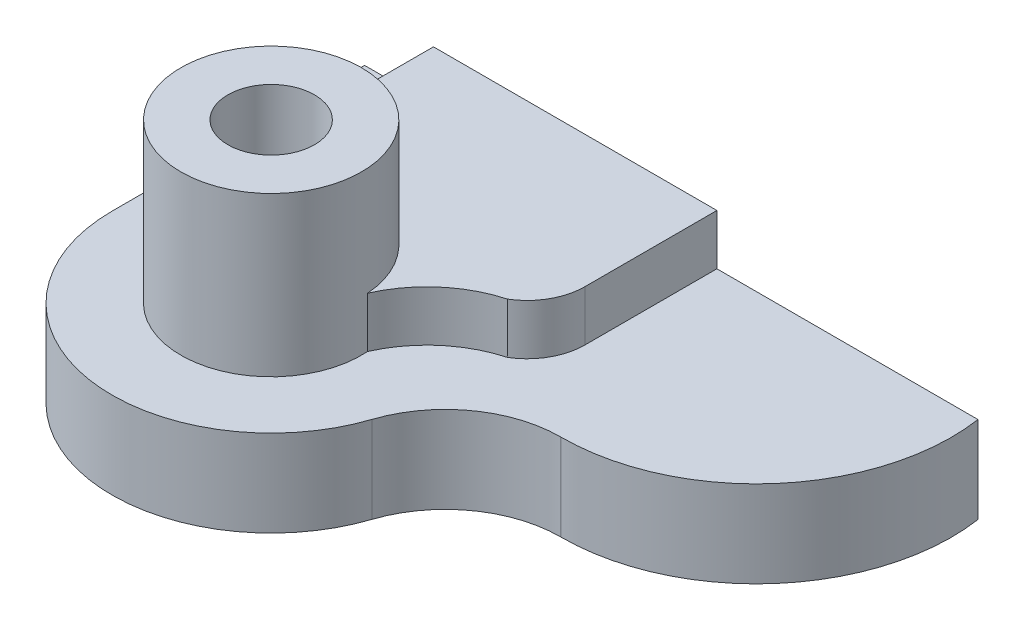
ISO-10303-21;
HEADER;
FILE_DESCRIPTION(('STEP AP214'),'2;1');
FILE_NAME('part.step','',(''),(''),'','','');
FILE_SCHEMA(('AUTOMOTIVE_DESIGN { 1 0 10303 214 1 1 1 1 }'));
ENDSEC;
DATA;
#1=APPLICATION_CONTEXT('core data for automotive mechanical design processes');
#2=APPLICATION_PROTOCOL_DEFINITION('international standard','automotive_design',2000,#1);
#3=PRODUCT_CONTEXT('',#1,'mechanical');
#4=PRODUCT('Part','Part','',(#3));
#5=PRODUCT_RELATED_PRODUCT_CATEGORY('part','',(#4));
#6=PRODUCT_DEFINITION_FORMATION('','',#4);
#7=PRODUCT_DEFINITION_CONTEXT('part definition',#1,'design');
#8=PRODUCT_DEFINITION('design','',#6,#7);
#9=PRODUCT_DEFINITION_SHAPE('','',#8);
#10=(LENGTH_UNIT() NAMED_UNIT(*) SI_UNIT(.MILLI.,.METRE.));
#11=(NAMED_UNIT(*) PLANE_ANGLE_UNIT() SI_UNIT($,.RADIAN.));
#12=(NAMED_UNIT(*) SI_UNIT($,.STERADIAN.) SOLID_ANGLE_UNIT());
#13=UNCERTAINTY_MEASURE_WITH_UNIT(LENGTH_MEASURE(1.E-05),#10,'distance_accuracy_value','');
#14=(GEOMETRIC_REPRESENTATION_CONTEXT(3) GLOBAL_UNCERTAINTY_ASSIGNED_CONTEXT((#13)) GLOBAL_UNIT_ASSIGNED_CONTEXT((#10,
#11,#12)) REPRESENTATION_CONTEXT('',''));
#15=CARTESIAN_POINT('',(0.,0.,0.));
#16=DIRECTION('',(0.,0.,1.));
#17=DIRECTION('',(1.,0.,0.));
#18=AXIS2_PLACEMENT_3D('',#15,#16,#17);
#19=CARTESIAN_POINT('',(36.1219032266776,12.,12.));
#20=DIRECTION('',(0.,1.,0.));
#21=DIRECTION('',(0.,0.,1.));
#22=AXIS2_PLACEMENT_3D('',#19,#20,#21);
#23=PLANE('',#22);
#24=CARTESIAN_POINT('',(0.,12.,0.));
#25=DIRECTION('',(0.,1.,0.));
#26=DIRECTION('',(0.,0.,1.));
#27=AXIS2_PLACEMENT_3D('',#24,#25,#26);
#28=CIRCLE('',#27,12.5129989979438);
#29=CARTESIAN_POINT('',(-12.5129989979438,12.,0.));
#30=VERTEX_POINT('',#29);
#31=CARTESIAN_POINT('',(12.4831428318669,12.,-0.863880177891194));
#32=VERTEX_POINT('',#31);
#33=EDGE_CURVE('E64',#30,#32,#28,.T.);
#34=ORIENTED_EDGE('',*,*,#33,.F.);
#35=DIRECTION('',(0.,0.,-1.));
#36=VECTOR('',#35,1.);
#37=CARTESIAN_POINT('',(-12.5129989979438,12.,0.));
#38=LINE('',#37,#36);
#39=CARTESIAN_POINT('',(-12.5129989979438,12.,-35.));
#40=VERTEX_POINT('',#39);
#41=EDGE_CURVE('E180',#30,#40,#38,.T.);
#42=ORIENTED_EDGE('',*,*,#41,.T.);
#43=DIRECTION('',(-1.,0.,0.));
#44=VECTOR('',#43,1.);
#45=CARTESIAN_POINT('',(-22.0629989979437,12.,-35.));
#46=LINE('',#45,#44);
#47=CARTESIAN_POINT('',(-22.0629989979437,12.,-35.));
#48=VERTEX_POINT('',#47);
#49=EDGE_CURVE('E203',#40,#48,#46,.T.);
#50=ORIENTED_EDGE('',*,*,#49,.T.);
#51=DIRECTION('',(0.,0.,1.));
#52=VECTOR('',#51,1.);
#53=CARTESIAN_POINT('',(-22.0629989979438,12.,0.));
#54=LINE('',#53,#52);
#55=CARTESIAN_POINT('',(-22.0629989979438,12.,0.));
#56=VERTEX_POINT('',#55);
#57=EDGE_CURVE('E204',#48,#56,#54,.T.);
#58=ORIENTED_EDGE('',*,*,#57,.T.);
#59=CARTESIAN_POINT('',(0.,12.,0.));
#60=DIRECTION('',(0.,1.,0.));
#61=DIRECTION('',(0.,0.,1.));
#62=AXIS2_PLACEMENT_3D('',#59,#60,#61);
#63=CIRCLE('',#62,22.0629989979438);
#64=CARTESIAN_POINT('',(20.9378539703891,12.,6.95573115480543));
#65=VERTEX_POINT('',#64);
#66=EDGE_CURVE('E206',#56,#65,#63,.T.);
#67=ORIENTED_EDGE('',*,*,#66,.T.);
#68=CARTESIAN_POINT('',(36.1219032266776,12.,12.));
#69=DIRECTION('',(0.,-1.,0.));
#70=DIRECTION('',(0.,0.,1.));
#71=AXIS2_PLACEMENT_3D('',#68,#69,#70);
#72=CIRCLE('',#71,16.);
#73=CARTESIAN_POINT('',(36.1219032266776,12.,-4.));
#74=VERTEX_POINT('',#73);
#75=EDGE_CURVE('E193',#65,#74,#72,.T.);
#76=ORIENTED_EDGE('',*,*,#75,.T.);
#77=DIRECTION('',(1.,0.,0.));
#78=VECTOR('',#77,1.);
#79=CARTESIAN_POINT('',(36.182547719487,12.,-4.));
#80=LINE('',#79,#78);
#81=CARTESIAN_POINT('',(36.182547719487,12.,-4.));
#82=VERTEX_POINT('',#81);
#83=EDGE_CURVE('E198',#74,#82,#80,.T.);
#84=ORIENTED_EDGE('',*,*,#83,.T.);
#85=CARTESIAN_POINT('',(36.182547719487,12.,-31.0451737169223));
#86=DIRECTION('',(0.,1.,0.));
#87=DIRECTION('',(0.,0.,1.));
#88=AXIS2_PLACEMENT_3D('',#85,#86,#87);
#89=CIRCLE('',#88,27.0451737169223);
#90=CARTESIAN_POINT('',(62.9370010020563,12.,-35.));
#91=VERTEX_POINT('',#90);
#92=EDGE_CURVE('E200',#82,#91,#89,.T.);
#93=ORIENTED_EDGE('',*,*,#92,.T.);
#94=CARTESIAN_POINT('',(26.7599670359934,12.,-35.));
#95=VERTEX_POINT('',#94);
#96=EDGE_CURVE('E205',#91,#95,#46,.T.);
#97=ORIENTED_EDGE('',*,*,#96,.T.);
#98=DIRECTION('',(0.,0.,-1.));
#99=VECTOR('',#98,1.);
#100=CARTESIAN_POINT('',(26.7599670359934,12.,0.));
#101=LINE('',#100,#99);
#102=CARTESIAN_POINT('',(26.7599670359934,12.,-16.7082857675377));
#103=VERTEX_POINT('',#102);
#104=EDGE_CURVE('E175',#103,#95,#101,.T.);
#105=ORIENTED_EDGE('',*,*,#104,.F.);
#106=CARTESIAN_POINT('',(18.7599670359934,12.,-16.7082857675377));
#107=DIRECTION('',(0.,1.,0.));
#108=DIRECTION('',(0.,0.,1.));
#109=AXIS2_PLACEMENT_3D('',#106,#107,#108);
#110=CIRCLE('',#109,8.);
#111=CARTESIAN_POINT('',(22.899922014398,12.,-9.86279288705179));
#112=VERTEX_POINT('',#111);
#113=EDGE_CURVE('E159',#103,#112,#110,.F.);
#114=ORIENTED_EDGE('',*,*,#113,.T.);
#115=CARTESIAN_POINT('',(27.1339469883604,12.,5.56682254949953));
#116=DIRECTION('',(0.,1.,0.));
#117=DIRECTION('',(0.,0.,1.));
#118=AXIS2_PLACEMENT_3D('',#115,#116,#117);
#119=CIRCLE('',#118,16.);
#120=EDGE_CURVE('E70',#32,#112,#119,.F.);
#121=ORIENTED_EDGE('',*,*,#120,.F.);
#122=EDGE_LOOP('',(#34,#42,#50,#58,#67,#76,#84,#93,#97,#105,#114,#121));
#123=FACE_BOUND('',#122,.T.);
#124=ADVANCED_FACE('F50',(#123),#23,.T.);
#125=CARTESIAN_POINT('',(36.1219032266776,12.,12.));
#126=DIRECTION('',(0.,-1.,0.));
#127=DIRECTION('',(0.,0.,-1.));
#128=AXIS2_PLACEMENT_3D('',#125,#126,#127);
#129=CYLINDRICAL_SURFACE('',#128,16.);
#130=CARTESIAN_POINT('',(36.1219032266776,0.,12.));
#131=DIRECTION('',(0.,-1.,0.));
#132=DIRECTION('',(0.,0.,1.));
#133=AXIS2_PLACEMENT_3D('',#130,#131,#132);
#134=CIRCLE('',#133,16.);
#135=CARTESIAN_POINT('',(20.9378539703891,0.,6.95573115480543));
#136=VERTEX_POINT('',#135);
#137=CARTESIAN_POINT('',(36.1219032266776,0.,-4.));
#138=VERTEX_POINT('',#137);
#139=EDGE_CURVE('E195',#136,#138,#134,.T.);
#140=ORIENTED_EDGE('',*,*,#139,.T.);
#141=DIRECTION('',(0.,-1.,0.));
#142=VECTOR('',#141,1.);
#143=CARTESIAN_POINT('',(36.1219032266776,12.,-4.));
#144=LINE('',#143,#142);
#145=EDGE_CURVE('E11',#74,#138,#144,.T.);
#146=ORIENTED_EDGE('',*,*,#145,.F.);
#147=ORIENTED_EDGE('',*,*,#75,.F.);
#148=DIRECTION('',(0.,-1.,0.));
#149=VECTOR('',#148,1.);
#150=CARTESIAN_POINT('',(20.9378539703891,12.,6.95573115480543));
#151=LINE('',#150,#149);
#152=EDGE_CURVE('E208',#65,#136,#151,.T.);
#153=ORIENTED_EDGE('',*,*,#152,.T.);
#154=EDGE_LOOP('',(#140,#146,#147,#153));
#155=FACE_BOUND('',#154,.T.);
#156=ADVANCED_FACE('F47',(#155),#129,.F.);
#157=CARTESIAN_POINT('',(36.182547719487,12.,-4.));
#158=DIRECTION('',(0.,0.,-1.));
#159=DIRECTION('',(-1.,0.,0.));
#160=AXIS2_PLACEMENT_3D('',#157,#158,#159);
#161=PLANE('',#160);
#162=DIRECTION('',(1.,0.,0.));
#163=VECTOR('',#162,1.);
#164=CARTESIAN_POINT('',(36.182547719487,0.,-4.));
#165=LINE('',#164,#163);
#166=CARTESIAN_POINT('',(36.182547719487,0.,-4.));
#167=VERTEX_POINT('',#166);
#168=EDGE_CURVE('E211',#138,#167,#165,.T.);
#169=ORIENTED_EDGE('',*,*,#168,.T.);
#170=DIRECTION('',(0.,-1.,0.));
#171=VECTOR('',#170,1.);
#172=CARTESIAN_POINT('',(36.182547719487,12.,-4.));
#173=LINE('',#172,#171);
#174=EDGE_CURVE('E54',#82,#167,#173,.T.);
#175=ORIENTED_EDGE('',*,*,#174,.F.);
#176=ORIENTED_EDGE('',*,*,#83,.F.);
#177=ORIENTED_EDGE('',*,*,#145,.T.);
#178=EDGE_LOOP('',(#169,#175,#176,#177));
#179=FACE_BOUND('',#178,.T.);
#180=ADVANCED_FACE('F276',(#179),#161,.F.);
#181=CARTESIAN_POINT('',(36.182547719487,12.,-31.0451737169223));
#182=DIRECTION('',(0.,-1.,0.));
#183=DIRECTION('',(0.,0.,-1.));
#184=AXIS2_PLACEMENT_3D('',#181,#182,#183);
#185=CYLINDRICAL_SURFACE('',#184,27.0451737169223);
#186=CARTESIAN_POINT('',(36.182547719487,0.,-31.0451737169223));
#187=DIRECTION('',(0.,1.,0.));
#188=DIRECTION('',(0.,0.,1.));
#189=AXIS2_PLACEMENT_3D('',#186,#187,#188);
#190=CIRCLE('',#189,27.0451737169223);
#191=CARTESIAN_POINT('',(62.9370010020563,0.,-35.));
#192=VERTEX_POINT('',#191);
#193=EDGE_CURVE('E213',#167,#192,#190,.T.);
#194=ORIENTED_EDGE('',*,*,#193,.T.);
#195=DIRECTION('',(0.,-1.,0.));
#196=VECTOR('',#195,1.);
#197=CARTESIAN_POINT('',(62.9370010020563,12.,-35.));
#198=LINE('',#197,#196);
#199=EDGE_CURVE('E227',#91,#192,#198,.T.);
#200=ORIENTED_EDGE('',*,*,#199,.F.);
#201=ORIENTED_EDGE('',*,*,#92,.F.);
#202=ORIENTED_EDGE('',*,*,#174,.T.);
#203=EDGE_LOOP('',(#194,#200,#201,#202));
#204=FACE_BOUND('',#203,.T.);
#205=ADVANCED_FACE('F231',(#204),#185,.T.);
#206=CARTESIAN_POINT('',(-22.0629989979437,12.,-35.));
#207=DIRECTION('',(0.,0.,1.));
#208=DIRECTION('',(1.,0.,0.));
#209=AXIS2_PLACEMENT_3D('',#206,#207,#208);
#210=PLANE('',#209);
#211=DIRECTION('',(-1.,0.,0.));
#212=VECTOR('',#211,1.);
#213=CARTESIAN_POINT('',(-22.0629989979437,0.,-35.));
#214=LINE('',#213,#212);
#215=CARTESIAN_POINT('',(-22.0629989979437,0.,-35.));
#216=VERTEX_POINT('',#215);
#217=EDGE_CURVE('E214',#192,#216,#214,.T.);
#218=ORIENTED_EDGE('',*,*,#217,.T.);
#219=DIRECTION('',(0.,-1.,0.));
#220=VECTOR('',#219,1.);
#221=CARTESIAN_POINT('',(-22.0629989979437,12.,-35.));
#222=LINE('',#221,#220);
#223=EDGE_CURVE('E223',#48,#216,#222,.T.);
#224=ORIENTED_EDGE('',*,*,#223,.F.);
#225=ORIENTED_EDGE('',*,*,#49,.F.);
#226=DIRECTION('',(0.,-1.,0.));
#227=VECTOR('',#226,1.);
#228=CARTESIAN_POINT('',(-12.5129989979438,19.,-35.));
#229=LINE('',#228,#227);
#230=CARTESIAN_POINT('',(-12.5129989979438,19.,-35.));
#231=VERTEX_POINT('',#230);
#232=EDGE_CURVE('E181',#231,#40,#229,.T.);
#233=ORIENTED_EDGE('',*,*,#232,.F.);
#234=DIRECTION('',(-1.,0.,0.));
#235=VECTOR('',#234,1.);
#236=CARTESIAN_POINT('',(0.,19.,-35.));
#237=LINE('',#236,#235);
#238=CARTESIAN_POINT('',(26.7599670359934,19.,-35.));
#239=VERTEX_POINT('',#238);
#240=EDGE_CURVE('E168',#239,#231,#237,.T.);
#241=ORIENTED_EDGE('',*,*,#240,.F.);
#242=DIRECTION('',(0.,-1.,0.));
#243=VECTOR('',#242,1.);
#244=CARTESIAN_POINT('',(26.7599670359934,19.,-35.));
#245=LINE('',#244,#243);
#246=EDGE_CURVE('E188',#239,#95,#245,.T.);
#247=ORIENTED_EDGE('',*,*,#246,.T.);
#248=ORIENTED_EDGE('',*,*,#96,.F.);
#249=ORIENTED_EDGE('',*,*,#199,.T.);
#250=EDGE_LOOP('',(#218,#224,#225,#233,#241,#247,#248,#249));
#251=FACE_BOUND('',#250,.T.);
#252=ADVANCED_FACE('F247',(#251),#210,.F.);
#253=CARTESIAN_POINT('',(-22.0629989979438,12.,0.));
#254=DIRECTION('',(1.,0.,0.));
#255=DIRECTION('',(0.,0.,-1.));
#256=AXIS2_PLACEMENT_3D('',#253,#254,#255);
#257=PLANE('',#256);
#258=DIRECTION('',(0.,0.,1.));
#259=VECTOR('',#258,1.);
#260=CARTESIAN_POINT('',(-22.0629989979438,0.,0.));
#261=LINE('',#260,#259);
#262=CARTESIAN_POINT('',(-22.0629989979438,0.,0.));
#263=VERTEX_POINT('',#262);
#264=EDGE_CURVE('E220',#216,#263,#261,.T.);
#265=ORIENTED_EDGE('',*,*,#264,.T.);
#266=DIRECTION('',(0.,-1.,0.));
#267=VECTOR('',#266,1.);
#268=CARTESIAN_POINT('',(-22.0629989979438,12.,0.));
#269=LINE('',#268,#267);
#270=EDGE_CURVE('E225',#56,#263,#269,.T.);
#271=ORIENTED_EDGE('',*,*,#270,.F.);
#272=ORIENTED_EDGE('',*,*,#57,.F.);
#273=ORIENTED_EDGE('',*,*,#223,.T.);
#274=EDGE_LOOP('',(#265,#271,#272,#273));
#275=FACE_BOUND('',#274,.T.);
#276=ADVANCED_FACE('F253',(#275),#257,.F.);
#277=CARTESIAN_POINT('',(0.,12.,0.));
#278=DIRECTION('',(0.,-1.,0.));
#279=DIRECTION('',(0.,0.,-1.));
#280=AXIS2_PLACEMENT_3D('',#277,#278,#279);
#281=CYLINDRICAL_SURFACE('',#280,22.0629989979438);
#282=CARTESIAN_POINT('',(0.,0.,0.));
#283=DIRECTION('',(0.,1.,0.));
#284=DIRECTION('',(0.,0.,1.));
#285=AXIS2_PLACEMENT_3D('',#282,#283,#284);
#286=CIRCLE('',#285,22.0629989979438);
#287=EDGE_CURVE('E197',#263,#136,#286,.T.);
#288=ORIENTED_EDGE('',*,*,#287,.T.);
#289=ORIENTED_EDGE('',*,*,#152,.F.);
#290=ORIENTED_EDGE('',*,*,#66,.F.);
#291=ORIENTED_EDGE('',*,*,#270,.T.);
#292=EDGE_LOOP('',(#288,#289,#290,#291));
#293=FACE_BOUND('',#292,.T.);
#294=ADVANCED_FACE('F281',(#293),#281,.T.);
#295=CARTESIAN_POINT('',(36.1219032266776,0.,12.));
#296=DIRECTION('',(0.,1.,0.));
#297=DIRECTION('',(0.,0.,1.));
#298=AXIS2_PLACEMENT_3D('',#295,#296,#297);
#299=PLANE('',#298);
#300=CARTESIAN_POINT('',(0.,0.,0.));
#301=DIRECTION('',(0.,1.,0.));
#302=DIRECTION('',(0.,0.,1.));
#303=AXIS2_PLACEMENT_3D('',#300,#301,#302);
#304=CIRCLE('',#303,6.);
#305=CARTESIAN_POINT('',(0.,0.,6.));
#306=VERTEX_POINT('',#305);
#307=EDGE_CURVE('E160',#306,#306,#304,.T.);
#308=ORIENTED_EDGE('',*,*,#307,.T.);
#309=EDGE_LOOP('',(#308));
#310=FACE_BOUND('',#309,.T.);
#311=ORIENTED_EDGE('',*,*,#139,.F.);
#312=ORIENTED_EDGE('',*,*,#287,.F.);
#313=ORIENTED_EDGE('',*,*,#264,.F.);
#314=ORIENTED_EDGE('',*,*,#217,.F.);
#315=ORIENTED_EDGE('',*,*,#193,.F.);
#316=ORIENTED_EDGE('',*,*,#168,.F.);
#317=EDGE_LOOP('',(#311,#312,#313,#314,#315,#316));
#318=FACE_BOUND('',#317,.T.);
#319=ADVANCED_FACE('F243',(#310,#318),#299,.F.);
#320=CARTESIAN_POINT('',(18.7599670359934,19.,-16.7082857675377));
#321=DIRECTION('',(0.,-1.,0.));
#322=DIRECTION('',(0.,0.,-1.));
#323=AXIS2_PLACEMENT_3D('',#320,#321,#322);
#324=CYLINDRICAL_SURFACE('',#323,8.);
#325=ORIENTED_EDGE('',*,*,#113,.F.);
#326=DIRECTION('',(0.,-1.,0.));
#327=VECTOR('',#326,1.);
#328=CARTESIAN_POINT('',(26.7599670359934,19.,-16.7082857675377));
#329=LINE('',#328,#327);
#330=CARTESIAN_POINT('',(26.7599670359934,19.,-16.7082857675377));
#331=VERTEX_POINT('',#330);
#332=EDGE_CURVE('E190',#331,#103,#329,.T.);
#333=ORIENTED_EDGE('',*,*,#332,.F.);
#334=CARTESIAN_POINT('',(18.7599670359934,19.,-16.7082857675377));
#335=DIRECTION('',(0.,1.,0.));
#336=DIRECTION('',(0.,0.,1.));
#337=AXIS2_PLACEMENT_3D('',#334,#335,#336);
#338=CIRCLE('',#337,8.);
#339=CARTESIAN_POINT('',(22.899922014398,19.,-9.86279288705179));
#340=VERTEX_POINT('',#339);
#341=EDGE_CURVE('E167',#331,#340,#338,.F.);
#342=ORIENTED_EDGE('',*,*,#341,.T.);
#343=DIRECTION('',(0.,-1.,0.));
#344=VECTOR('',#343,1.);
#345=CARTESIAN_POINT('',(22.899922014398,19.,-9.86279288705179));
#346=LINE('',#345,#344);
#347=EDGE_CURVE('E139',#340,#112,#346,.T.);
#348=ORIENTED_EDGE('',*,*,#347,.T.);
#349=EDGE_LOOP('',(#325,#333,#342,#348));
#350=FACE_BOUND('',#349,.T.);
#351=ADVANCED_FACE('F267',(#350),#324,.T.);
#352=CARTESIAN_POINT('',(26.7599670359934,19.,0.));
#353=DIRECTION('',(-1.,0.,0.));
#354=DIRECTION('',(0.,0.,1.));
#355=AXIS2_PLACEMENT_3D('',#352,#353,#354);
#356=PLANE('',#355);
#357=ORIENTED_EDGE('',*,*,#104,.T.);
#358=ORIENTED_EDGE('',*,*,#246,.F.);
#359=DIRECTION('',(0.,0.,-1.));
#360=VECTOR('',#359,1.);
#361=CARTESIAN_POINT('',(26.7599670359934,19.,0.));
#362=LINE('',#361,#360);
#363=EDGE_CURVE('E169',#331,#239,#362,.T.);
#364=ORIENTED_EDGE('',*,*,#363,.F.);
#365=ORIENTED_EDGE('',*,*,#332,.T.);
#366=EDGE_LOOP('',(#357,#358,#364,#365));
#367=FACE_BOUND('',#366,.T.);
#368=ADVANCED_FACE('F261',(#367),#356,.F.);
#369=CARTESIAN_POINT('',(-12.5129989979438,19.,0.));
#370=DIRECTION('',(-1.,0.,0.));
#371=DIRECTION('',(0.,0.,1.));
#372=AXIS2_PLACEMENT_3D('',#369,#370,#371);
#373=PLANE('',#372);
#374=ORIENTED_EDGE('',*,*,#41,.F.);
#375=DIRECTION('',(0.,-1.,0.));
#376=VECTOR('',#375,1.);
#377=CARTESIAN_POINT('',(-12.5129989979438,19.,0.));
#378=LINE('',#377,#376);
#379=CARTESIAN_POINT('',(-12.5129989979438,19.,0.));
#380=VERTEX_POINT('',#379);
#381=EDGE_CURVE('E151',#380,#30,#378,.T.);
#382=ORIENTED_EDGE('',*,*,#381,.F.);
#383=DIRECTION('',(0.,0.,-1.));
#384=VECTOR('',#383,1.);
#385=CARTESIAN_POINT('',(-12.5129989979438,19.,0.));
#386=LINE('',#385,#384);
#387=EDGE_CURVE('E145',#380,#231,#386,.T.);
#388=ORIENTED_EDGE('',*,*,#387,.T.);
#389=ORIENTED_EDGE('',*,*,#232,.T.);
#390=EDGE_LOOP('',(#374,#382,#388,#389));
#391=FACE_BOUND('',#390,.T.);
#392=ADVANCED_FACE('F259',(#391),#373,.T.);
#393=CARTESIAN_POINT('',(0.,19.,0.));
#394=DIRECTION('',(0.,-1.,0.));
#395=DIRECTION('',(0.,0.,-1.));
#396=AXIS2_PLACEMENT_3D('',#393,#394,#395);
#397=CYLINDRICAL_SURFACE('',#396,12.5129989979438);
#398=ORIENTED_EDGE('',*,*,#33,.T.);
#399=DIRECTION('',(0.,-1.,0.));
#400=VECTOR('',#399,1.);
#401=CARTESIAN_POINT('',(12.4831428318669,19.,-0.863880177891194));
#402=LINE('',#401,#400);
#403=CARTESIAN_POINT('',(12.4831428318669,19.,-0.863880177891194));
#404=VERTEX_POINT('',#403);
#405=EDGE_CURVE('E140',#404,#32,#402,.T.);
#406=ORIENTED_EDGE('',*,*,#405,.F.);
#407=CARTESIAN_POINT('',(0.,19.,0.));
#408=DIRECTION('',(0.,1.,0.));
#409=DIRECTION('',(0.,0.,1.));
#410=AXIS2_PLACEMENT_3D('',#407,#408,#409);
#411=CIRCLE('',#410,12.5129989979438);
#412=EDGE_CURVE('E147',#404,#380,#411,.T.);
#413=ORIENTED_EDGE('',*,*,#412,.T.);
#414=ORIENTED_EDGE('',*,*,#381,.T.);
#415=EDGE_LOOP('',(#398,#406,#413,#414));
#416=FACE_BOUND('',#415,.T.);
#417=CARTESIAN_POINT('',(0.,34.,0.));
#418=DIRECTION('',(0.,1.,0.));
#419=DIRECTION('',(0.,0.,1.));
#420=AXIS2_PLACEMENT_3D('',#417,#418,#419);
#421=CIRCLE('',#420,12.5129989979438);
#422=CARTESIAN_POINT('',(0.,34.,12.5129989979438));
#423=VERTEX_POINT('',#422);
#424=EDGE_CURVE('E156',#423,#423,#421,.T.);
#425=ORIENTED_EDGE('',*,*,#424,.F.);
#426=EDGE_LOOP('',(#425));
#427=FACE_BOUND('',#426,.T.);
#428=ADVANCED_FACE('F146',(#416,#427),#397,.T.);
#429=CARTESIAN_POINT('',(27.1339469883604,19.,5.56682254949953));
#430=DIRECTION('',(0.,-1.,0.));
#431=DIRECTION('',(0.,0.,-1.));
#432=AXIS2_PLACEMENT_3D('',#429,#430,#431);
#433=CYLINDRICAL_SURFACE('',#432,16.);
#434=ORIENTED_EDGE('',*,*,#120,.T.);
#435=ORIENTED_EDGE('',*,*,#347,.F.);
#436=CARTESIAN_POINT('',(27.1339469883604,19.,5.56682254949953));
#437=DIRECTION('',(0.,1.,0.));
#438=DIRECTION('',(0.,0.,1.));
#439=AXIS2_PLACEMENT_3D('',#436,#437,#438);
#440=CIRCLE('',#439,16.);
#441=EDGE_CURVE('E135',#404,#340,#440,.F.);
#442=ORIENTED_EDGE('',*,*,#441,.F.);
#443=ORIENTED_EDGE('',*,*,#405,.T.);
#444=EDGE_LOOP('',(#434,#435,#442,#443));
#445=FACE_BOUND('',#444,.T.);
#446=ADVANCED_FACE('F137',(#445),#433,.F.);
#447=CARTESIAN_POINT('',(0.,19.,0.));
#448=DIRECTION('',(0.,1.,0.));
#449=DIRECTION('',(0.,0.,1.));
#450=AXIS2_PLACEMENT_3D('',#447,#448,#449);
#451=PLANE('',#450);
#452=ORIENTED_EDGE('',*,*,#412,.F.);
#453=ORIENTED_EDGE('',*,*,#441,.T.);
#454=ORIENTED_EDGE('',*,*,#341,.F.);
#455=ORIENTED_EDGE('',*,*,#363,.T.);
#456=ORIENTED_EDGE('',*,*,#240,.T.);
#457=ORIENTED_EDGE('',*,*,#387,.F.);
#458=EDGE_LOOP('',(#452,#453,#454,#455,#456,#457));
#459=FACE_BOUND('',#458,.T.);
#460=ADVANCED_FACE('F152',(#459),#451,.T.);
#461=CARTESIAN_POINT('',(0.,34.,0.));
#462=DIRECTION('',(0.,1.,0.));
#463=DIRECTION('',(0.,0.,1.));
#464=AXIS2_PLACEMENT_3D('',#461,#462,#463);
#465=PLANE('',#464);
#466=CARTESIAN_POINT('',(0.,34.,0.));
#467=DIRECTION('',(0.,1.,0.));
#468=DIRECTION('',(0.,0.,1.));
#469=AXIS2_PLACEMENT_3D('',#466,#467,#468);
#470=CIRCLE('',#469,6.);
#471=CARTESIAN_POINT('',(0.,34.,6.));
#472=VERTEX_POINT('',#471);
#473=EDGE_CURVE('E162',#472,#472,#470,.T.);
#474=ORIENTED_EDGE('',*,*,#473,.F.);
#475=EDGE_LOOP('',(#474));
#476=FACE_BOUND('',#475,.T.);
#477=ORIENTED_EDGE('',*,*,#424,.T.);
#478=EDGE_LOOP('',(#477));
#479=FACE_BOUND('',#478,.T.);
#480=ADVANCED_FACE('F335',(#476,#479),#465,.T.);
#481=CARTESIAN_POINT('',(0.,-34.,0.));
#482=DIRECTION('',(0.,1.,0.));
#483=DIRECTION('',(0.,0.,1.));
#484=AXIS2_PLACEMENT_3D('',#481,#482,#483);
#485=CYLINDRICAL_SURFACE('',#484,6.);
#486=ORIENTED_EDGE('',*,*,#473,.T.);
#487=EDGE_LOOP('',(#486));
#488=FACE_BOUND('',#487,.T.);
#489=ORIENTED_EDGE('',*,*,#307,.F.);
#490=EDGE_LOOP('',(#489));
#491=FACE_BOUND('',#490,.T.);
#492=ADVANCED_FACE('F341',(#488,#491),#485,.F.);
#493=CLOSED_SHELL('',(#124,#156,#180,#205,#252,#276,#294,#319,#351,#368,#392,#428,#446,#460,
#480,#492));
#494=MANIFOLD_SOLID_BREP('B2',#493);
#495=ADVANCED_BREP_SHAPE_REPRESENTATION('',(#18,#494),#14);
#496=SHAPE_DEFINITION_REPRESENTATION(#9,#495);
ENDSEC;
END-ISO-10303-21;
